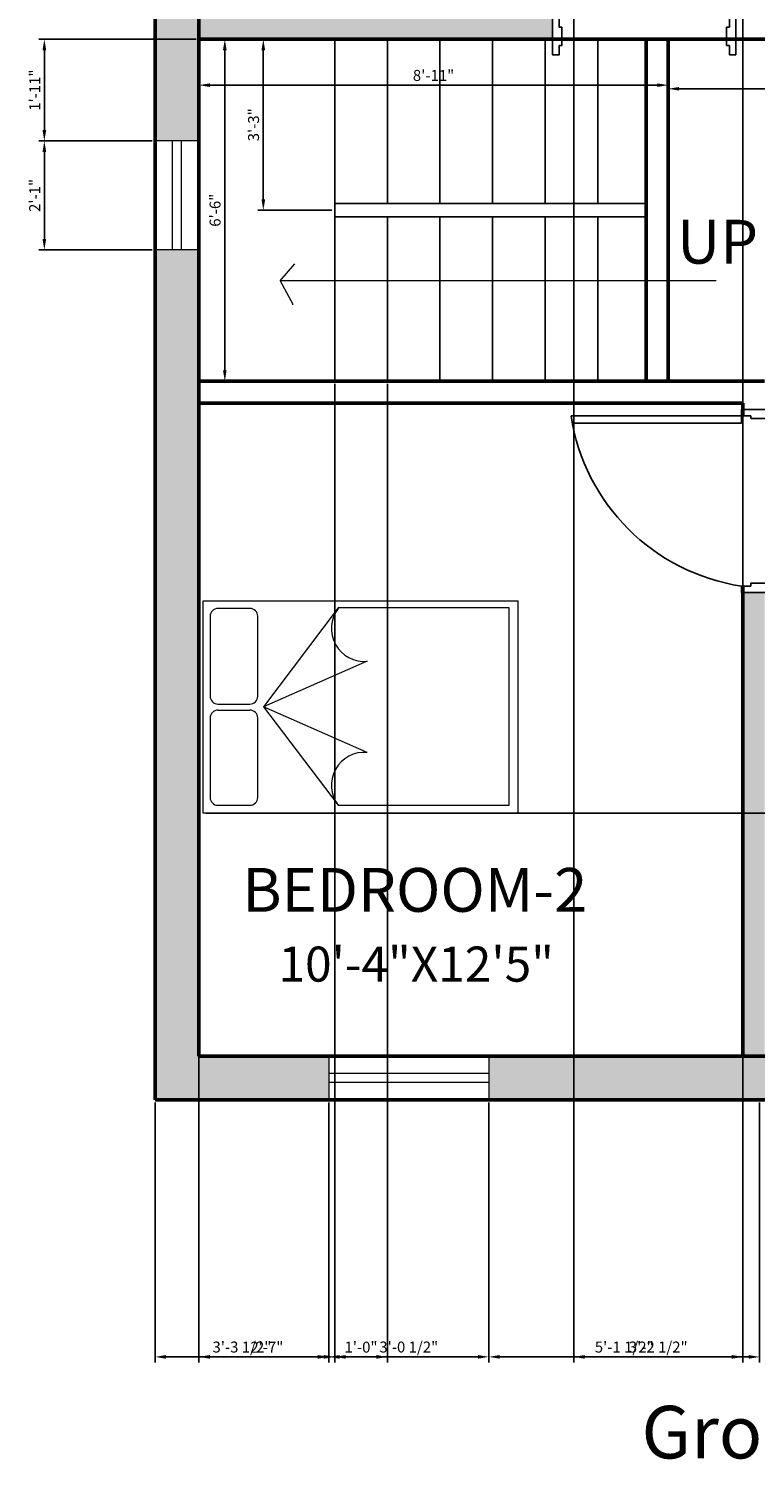
# Model space of a CAD drawing. Units: inches. Extents: x 3578 to 3951, y 1675 to 2189.
# Tile 1 of 4: x 3580 to 3746, y 1675 to 2001. Entities that reach past the tile are written whole.
import ezdxf

# ---------------------------------------------------------------- set-up
doc = ezdxf.new("R2010")
doc.units = ezdxf.units.IN
for name, color, linetype, lineweight in [('A-ANNO-DIMS', 2, 'Continuous', 18), ('A-ANNO-SYMB', 7, 'Continuous', 18), ('A-ANNO-TEXT', 7, 'Continuous', 25), ('A-AREA-IDEN', 7, 'Continuous', 25), ('A-DOOR', 3, 'Continuous', 25), ('A-FLOR-STRS', 7, 'Continuous', 25), ('A-FURN', 8, 'Continuous', 18), ('A-GLAZ', 4, 'Continuous', 18), ('A-WALL', 7, 'Continuous', 50), ('A-WALL-PATT', 8, 'Continuous', 13)]:
    doc.layers.add(name, color=color, linetype=linetype, lineweight=lineweight)
doc.styles.get("Standard").update_dxf_attribs({"font": 'arial.ttf'})
doc.dimstyles.new('ISO-25', dxfattribs={"dimtxt": 2.5, "dimasz": 2.5, "dimexe": 1.25, "dimexo": 0.625, "dimtad": 1, "dimdec": 0, "dimlunit": 4, "dimtxsty": 'Standard', "dimcen": 2.5, "dimadec": 0, "dimazin": 0, "dimtfac": 1, "dimtdec": 0, "dimtmove": 0, "dimatfit": 3, "dimfxl": 1, "dimarcsym": 0})

# ---------------------------------------------------------------- blocks, each defined once
blk = doc.blocks.new('A$C36772BAF')
for p, q in [((0, 0), (0, 2)), ((0, 2), (1.35, 2)), ((1.35, 2), (1.35, 0)), ((0.6051, 1.9554), (0.1004, 1.9554)), ((1.2508, 1.9554), (0.7437, 1.9554)), ((0.0504, 1.9054), (0.0504, 1.7024)), ((0.6551, 1.9054), (0.6551, 1.7024)), ((0.6937, 1.9054), (0.6937, 1.7024)), ((1.3008, 1.7024), (1.3008, 1.9054)), ((0.1004, 1.6524), (0.6051, 1.6524)), ((0.7437, 1.6524), (1.2508, 1.6524)), ((0.6756, 1.6168), (0.0504, 1.1415)), ((0.386, 0.9573), (0.6756, 1.6168)), ((0.9651, 0.9573), (0.6756, 1.6168)), ((1.305, 1.1415), (0.6756, 1.6168)), ((0.0504, 1.1415), (0.0504, 0.0572)), ((1.305, 0.0572), (1.305, 1.1415)), ((0, 0), (1.35, 0)), ((0.0504, 0.0572), (1.305, 0.0572))]:
    blk.add_line(p, q)
for centre, radius, start, end in [((0.1004, 1.9054), 0.05, 90, 180), ((0.6051, 1.9054), 0.05, 0, 90), ((0.7437, 1.9054), 0.05, 90, 180), ((1.2508, 1.9054), 0.05, 0, 90), ((0.1004, 1.7024), 0.05, 180, 270), ((0.6051, 1.7024), 0.05, 270, 0), ((0.7437, 1.7024), 0.05, 180, 270), ((1.2508, 1.7024), 0.05, 270, 0), ((0.1778, 0.9758), 0.2091, 354.93576, 127.55915), ((1.1733, 0.9758), 0.2091, 52.44085, 185.06424)]:
    blk.add_arc(centre, radius, start, end)
blk = doc.blocks.new('A$C40E8097C')
for p, q in [((33.6, 192), (33.6, 1074.8)), ((72, 192), (72, 1068.3)), ((0, 192), (0, 0)), ((33.6, 192), (0, 192)), ((33.6, 144), (33.6, 192)), ((48, 144), (33.6, 144)), ((48, 48), (48, 144)), ((33.6, 0), (33.6, 48)), ((33.6, 48), (48, 48)), ((0, 0), (33.6, 0))]:
    blk.add_line(p, q)
blk.add_lwpolyline([(33.6, 192), (72, 192)])
blk.add_lwpolyline([(950, 192), (950, 0), (916.4, 0), (916.4, 48), (902, 48), (902, 144), (916.4, 144), (916.4, 192)], close=True)
blk.add_arc((-123.6, 34.8), 1051.8, 8.59637, 81.40363)
blk = doc.blocks.new('*D8')
at = {"layer": 'A-ANNO-DIMS', "color": 0, "lineweight": -2, "transparency": 16777216}
for p, q in [((3619.18, 1998.14), (3619.18, 1987.06)), ((3726.18, 1998.14), (3726.18, 1987.06)), ((3621.68, 1988.31), (3723.68, 1988.31))]:
    blk.add_line(p, q, dxfattribs=at)
at = {"layer": 'A-ANNO-DIMS', "color": 0, "transparency": 16777216}
for points in [[(3621.68, 1988.72), (3621.68, 1987.89), (3619.18, 1988.31)], [(3723.68, 1988.72), (3723.68, 1987.89), (3726.18, 1988.31)]]:
    blk.add_solid(points, dxfattribs=at)
at = {"layer": 'Defpoints', "color": 0, "transparency": 16777216}
for p in [(3619.18, 1998.77), (3726.18, 1998.77), (3726.18, 1988.31)]:
    blk.add_point(p, dxfattribs=at)
at = {"layer": 'A-ANNO-DIMS', "color": 0, "transparency": 16777216, "insert": (3672.68, 1990.21), "char_height": 2.5, "attachment_point": 5}
blk.add_mtext('8\'-11"', dxfattribs=at)
blk = doc.blocks.new('*D9')
at = {"layer": 'A-ANNO-DIMS', "color": 0, "lineweight": -2, "transparency": 16777216}
for p, q in [((3649.51, 1998.77), (3632.61, 1998.77)), ((3633.86, 1996.27), (3633.86, 1962.27)), ((3649.51, 1959.77), (3632.61, 1959.77))]:
    blk.add_line(p, q, dxfattribs=at)
at = {"layer": 'A-ANNO-DIMS', "color": 0, "transparency": 16777216}
for points in [[(3633.44, 1996.27), (3634.28, 1996.27), (3633.86, 1998.77)], [(3633.44, 1962.27), (3634.28, 1962.27), (3633.86, 1959.77)]]:
    blk.add_solid(points, dxfattribs=at)
at = {"layer": 'Defpoints', "color": 0, "transparency": 16777216}
for p in [(3650.14, 1998.77), (3633.86, 1959.77), (3650.14, 1959.77)]:
    blk.add_point(p, dxfattribs=at)
at = {"layer": 'A-ANNO-DIMS', "color": 0, "transparency": 16777216, "insert": (3631.96, 1979.27), "char_height": 2.5, "attachment_point": 5, "rotation": 90}
blk.add_mtext('3\'-3"', dxfattribs=at)
blk = doc.blocks.new('*D10')
at = {"layer": 'A-ANNO-DIMS', "color": 0, "lineweight": -2, "transparency": 16777216}
for p, q in [((3619.8, 1998.77), (3626.33, 1998.77)), ((3625.08, 1996.27), (3625.08, 1923.27)), ((3619.8, 1920.77), (3626.33, 1920.77))]:
    blk.add_line(p, q, dxfattribs=at)
at = {"layer": 'A-ANNO-DIMS', "color": 0, "transparency": 16777216}
for points in [[(3624.66, 1996.27), (3625.5, 1996.27), (3625.08, 1998.77)], [(3624.66, 1923.27), (3625.5, 1923.27), (3625.08, 1920.77)]]:
    blk.add_solid(points, dxfattribs=at)
at = {"layer": 'Defpoints', "color": 0, "transparency": 16777216}
for p in [(3619.18, 1998.77), (3619.18, 1920.77), (3625.08, 1920.77)]:
    blk.add_point(p, dxfattribs=at)
at = {"layer": 'A-ANNO-DIMS', "color": 0, "transparency": 16777216, "insert": (3623.18, 1959.77), "char_height": 2.5, "attachment_point": 5, "rotation": 90}
blk.add_mtext('6\'-6"', dxfattribs=at)
blk = doc.blocks.new('*D12')
at = {"layer": 'A-ANNO-DIMS', "color": 0, "lineweight": -2, "transparency": 16777216}
for p, q in [((3726.18, 1987.68), (3726.18, 1986.23)), ((3728.68, 1987.48), (3821.68, 1987.48)), ((3824.18, 1987.68), (3824.18, 1986.23))]:
    blk.add_line(p, q, dxfattribs=at)
at = {"layer": 'A-ANNO-DIMS', "color": 0, "transparency": 16777216}
for points in [[(3728.68, 1987.9), (3728.68, 1987.07), (3726.18, 1987.48)], [(3821.68, 1987.9), (3821.68, 1987.07), (3824.18, 1987.48)]]:
    blk.add_solid(points, dxfattribs=at)
at = {"layer": 'Defpoints', "color": 0, "transparency": 16777216}
for p in [(3726.18, 1988.31), (3824.18, 1988.31), (3824.18, 1987.48)]:
    blk.add_point(p, dxfattribs=at)
at = {"layer": 'A-ANNO-DIMS', "color": 0, "transparency": 16777216, "insert": (3775.18, 1989.38), "char_height": 2.5, "attachment_point": 5}
blk.add_mtext('8\'-2"', dxfattribs=at)
blk = doc.blocks.new('*D29')
at = {"layer": 'A-ANNO-DIMS', "color": 0, "lineweight": -2, "transparency": 16777216}
for p, q in [((3618.55, 1998.77), (3582.68, 1998.77)), ((3583.93, 1996.27), (3583.93, 1978.07)), ((3608.55, 1975.57), (3582.68, 1975.57))]:
    blk.add_line(p, q, dxfattribs=at)
at = {"layer": 'A-ANNO-DIMS', "color": 0, "transparency": 16777216}
for points in [[(3583.51, 1996.27), (3584.35, 1996.27), (3583.93, 1998.77)], [(3583.51, 1978.07), (3584.35, 1978.07), (3583.93, 1975.57)]]:
    blk.add_solid(points, dxfattribs=at)
at = {"layer": 'Defpoints', "color": 0, "transparency": 16777216}
for p in [(3619.18, 1998.77), (3583.93, 1975.57), (3609.18, 1975.57)]:
    blk.add_point(p, dxfattribs=at)
at = {"layer": 'A-ANNO-DIMS', "color": 0, "transparency": 16777216, "insert": (3582.05, 1987.17), "char_height": 2.5, "attachment_point": 5, "rotation": 90}
blk.add_mtext('1\'-11"', dxfattribs=at)
blk = doc.blocks.new('*D30')
at = {"layer": 'A-ANNO-DIMS', "color": 0, "lineweight": -2, "transparency": 16777216}
for p, q in [((3608.55, 1975.57), (3582.68, 1975.57)), ((3583.93, 1973.07), (3583.93, 1953.21)), ((3608.55, 1950.71), (3582.68, 1950.71))]:
    blk.add_line(p, q, dxfattribs=at)
at = {"layer": 'A-ANNO-DIMS', "color": 0, "transparency": 16777216}
for points in [[(3583.51, 1973.07), (3584.35, 1973.07), (3583.93, 1975.57)], [(3583.51, 1953.21), (3584.35, 1953.21), (3583.93, 1950.71)]]:
    blk.add_solid(points, dxfattribs=at)
at = {"layer": 'Defpoints', "color": 0, "transparency": 16777216}
for p in [(3609.18, 1975.57), (3583.93, 1950.71), (3609.18, 1950.71)]:
    blk.add_point(p, dxfattribs=at)
at = {"layer": 'A-ANNO-DIMS', "color": 0, "transparency": 16777216, "insert": (3582.05, 1963.14), "char_height": 2.5, "attachment_point": 5, "rotation": 90}
blk.add_mtext('2\'-1"', dxfattribs=at)
blk = doc.blocks.new('*D37')
at = {"layer": 'A-ANNO-DIMS', "color": 0, "lineweight": -2, "transparency": 16777216}
for p, q in [((3609.18, 1756.14), (3609.18, 1696.88)), ((3648.78, 1756.14), (3648.78, 1696.88)), ((3611.68, 1698.13), (3646.28, 1698.13))]:
    blk.add_line(p, q, dxfattribs=at)
at = {"layer": 'A-ANNO-DIMS', "color": 0, "transparency": 16777216}
for points in [[(3611.68, 1698.55), (3611.68, 1697.71), (3609.18, 1698.13)], [(3646.28, 1698.55), (3646.28, 1697.71), (3648.78, 1698.13)]]:
    blk.add_solid(points, dxfattribs=at)
at = {"layer": 'Defpoints', "color": 0, "transparency": 16777216}
for p in [(3609.18, 1756.77), (3648.78, 1756.77), (3648.78, 1698.13)]:
    blk.add_point(p, dxfattribs=at)
at = {"layer": 'A-ANNO-DIMS', "color": 0, "transparency": 16777216, "insert": (3628.98, 1700.05), "char_height": 2.5, "attachment_point": 5}
blk.add_mtext('3\'-3 1/2"', dxfattribs=at)
blk = doc.blocks.new('*D38')
at = {"layer": 'A-ANNO-DIMS', "color": 0, "lineweight": -2, "transparency": 16777216}
for p, q in [((3648.78, 1756.14), (3648.78, 1696.88)), ((3685.29, 1756.14), (3685.29, 1696.88)), ((3651.28, 1698.13), (3682.79, 1698.13))]:
    blk.add_line(p, q, dxfattribs=at)
at = {"layer": 'A-ANNO-DIMS', "color": 0, "transparency": 16777216}
for points in [[(3651.28, 1698.55), (3651.28, 1697.71), (3648.78, 1698.13)], [(3682.79, 1698.55), (3682.79, 1697.71), (3685.29, 1698.13)]]:
    blk.add_solid(points, dxfattribs=at)
at = {"layer": 'Defpoints', "color": 0, "transparency": 16777216}
for p in [(3648.78, 1756.77), (3685.29, 1756.77), (3685.29, 1698.13)]:
    blk.add_point(p, dxfattribs=at)
at = {"layer": 'A-ANNO-DIMS', "color": 0, "transparency": 16777216, "insert": (3667.03, 1700.05), "char_height": 2.5, "attachment_point": 5}
blk.add_mtext('3\'-0 1/2"', dxfattribs=at)
blk = doc.blocks.new('*D39')
at = {"layer": 'A-ANNO-DIMS', "color": 0, "lineweight": -2, "transparency": 16777216}
for p, q in [((3685.29, 1756.14), (3685.29, 1696.88)), ((3747.04, 1756.14), (3747.04, 1696.88)), ((3687.79, 1698.13), (3744.54, 1698.13))]:
    blk.add_line(p, q, dxfattribs=at)
at = {"layer": 'A-ANNO-DIMS', "color": 0, "transparency": 16777216}
for points in [[(3687.79, 1698.55), (3687.79, 1697.71), (3685.29, 1698.13)], [(3744.54, 1698.55), (3744.54, 1697.71), (3747.04, 1698.13)]]:
    blk.add_solid(points, dxfattribs=at)
at = {"layer": 'Defpoints', "color": 0, "transparency": 16777216}
for p in [(3685.29, 1756.77), (3747.04, 1756.77), (3747.04, 1698.13)]:
    blk.add_point(p, dxfattribs=at)
at = {"layer": 'A-ANNO-DIMS', "color": 0, "transparency": 16777216, "insert": (3716.16, 1700.05), "char_height": 2.5, "attachment_point": 5}
blk.add_mtext('5\'-1 1/2"', dxfattribs=at)
blk = doc.blocks.new('*D49')
at = {"layer": 'A-ANNO-DIMS', "color": 0, "lineweight": -2, "transparency": 16777216}
for p, q in [((3619.18, 1920.14), (3619.18, 1696.88)), ((3650.14, 1920.14), (3650.14, 1696.88)), ((3621.68, 1698.13), (3647.64, 1698.13))]:
    blk.add_line(p, q, dxfattribs=at)
at = {"layer": 'A-ANNO-DIMS', "color": 0, "transparency": 16777216}
for points in [[(3621.68, 1698.55), (3621.68, 1697.71), (3619.18, 1698.13)], [(3647.64, 1698.55), (3647.64, 1697.71), (3650.14, 1698.13)]]:
    blk.add_solid(points, dxfattribs=at)
at = {"layer": 'Defpoints', "color": 0, "transparency": 16777216}
for p in [(3619.18, 1920.77), (3650.14, 1920.77), (3650.14, 1698.13)]:
    blk.add_point(p, dxfattribs=at)
at = {"layer": 'A-ANNO-DIMS', "color": 0, "transparency": 16777216, "insert": (3634.66, 1700.01), "char_height": 2.5, "attachment_point": 5}
blk.add_mtext('2\'-7"', dxfattribs=at)
blk = doc.blocks.new('*D50')
at = {"layer": 'A-ANNO-DIMS', "color": 0, "lineweight": -2, "transparency": 16777216}
for p, q in [((3650.14, 1920.14), (3650.14, 1696.88)), ((3662.14, 1920.14), (3662.14, 1696.88)), ((3652.64, 1698.13), (3659.64, 1698.13))]:
    blk.add_line(p, q, dxfattribs=at)
at = {"layer": 'A-ANNO-DIMS', "color": 0, "transparency": 16777216}
for points in [[(3652.64, 1698.55), (3652.64, 1697.71), (3650.14, 1698.13)], [(3659.64, 1698.55), (3659.64, 1697.71), (3662.14, 1698.13)]]:
    blk.add_solid(points, dxfattribs=at)
at = {"layer": 'Defpoints', "color": 0, "transparency": 16777216}
for p in [(3650.14, 1920.77), (3662.14, 1920.77), (3662.14, 1698.13)]:
    blk.add_point(p, dxfattribs=at)
at = {"layer": 'A-ANNO-DIMS', "color": 0, "transparency": 16777216, "insert": (3656.14, 1700.03), "char_height": 2.5, "attachment_point": 5}
blk.add_mtext('1\'-0"', dxfattribs=at)
blk = doc.blocks.new('*D54')
at = {"layer": 'A-ANNO-DIMS', "color": 0, "lineweight": -2, "transparency": 16777216}
for p, q in [((3704.64, 2107.33), (3704.64, 1696.88)), ((3743.18, 2098.14), (3743.18, 1696.88)), ((3740.68, 1698.13), (3707.14, 1698.13))]:
    blk.add_line(p, q, dxfattribs=at)
at = {"layer": 'A-ANNO-DIMS', "color": 0, "transparency": 16777216}
for points in [[(3707.14, 1698.55), (3707.14, 1697.71), (3704.64, 1698.13)], [(3740.68, 1698.55), (3740.68, 1697.71), (3743.18, 1698.13)]]:
    blk.add_solid(points, dxfattribs=at)
at = {"layer": 'Defpoints', "color": 0, "transparency": 16777216}
for p in [(3704.64, 2107.95), (3743.18, 2098.77), (3704.64, 1698.13)]:
    blk.add_point(p, dxfattribs=at)
at = {"layer": 'A-ANNO-DIMS', "color": 0, "transparency": 16777216, "insert": (3723.91, 1700.05), "char_height": 2.5, "attachment_point": 5}
blk.add_mtext('3\'-2 1/2"', dxfattribs=at)
blk = doc.blocks.new('*D57')
at = {"layer": 'A-ANNO-DIMS', "color": 0, "lineweight": -2, "transparency": 16777216}
for p, q in [((3620.74, 1822.18), (3936.33, 1822.18)), ((3935.08, 1769.27), (3935.08, 1819.68)), ((3619.8, 1766.77), (3936.33, 1766.77))]:
    blk.add_line(p, q, dxfattribs=at)
at = {"layer": 'A-ANNO-DIMS', "color": 0, "transparency": 16777216}
for points in [[(3934.66, 1819.68), (3935.5, 1819.68), (3935.08, 1822.18)], [(3934.66, 1769.27), (3935.5, 1769.27), (3935.08, 1766.77)]]:
    blk.add_solid(points, dxfattribs=at)
at = {"layer": 'Defpoints', "color": 0, "transparency": 16777216}
for p in [(3620.11, 1822.18), (3935.08, 1822.18), (3619.18, 1766.77)]:
    blk.add_point(p, dxfattribs=at)
at = {"layer": 'A-ANNO-DIMS', "color": 0, "transparency": 16777216, "insert": (3933.16, 1794.47), "char_height": 2.5, "attachment_point": 5, "rotation": 90}
blk.add_mtext('4\'-7 1/2"', dxfattribs=at)

msp = doc.modelspace()

# ---------------------------------------------------------------- hatches: boundary and pattern name
at = {"layer": 'A-WALL-PATT'}
h = msp.add_hatch(color=256, dxfattribs=at)
h.dxf.hatch_style = 1
h.paths.add_polyline_path([(3619.18, 1950.71), (3609.18, 1950.71), (3609.18, 1756.77), (3648.78, 1756.77), (3648.78, 1766.77), (3619.18, 1766.77)])
h.paths.add_polyline_path([(3619.18, 2068.71), (3609.18, 2068.71), (3609.18, 1975.57), (3619.18, 1975.57), (3619.18, 1998.77)])
h.paths.add_polyline_path([(3619.18, 2130.77), (3647.07, 2130.77), (3647.07, 2140.77), (3609.18, 2140.77), (3609.18, 2104.48), (3619.18, 2104.48)])
h.paths.add_polyline_path([(3909.18, 2140.77), (3713.13, 2140.77), (3713.13, 2130.77), (3899.18, 2130.77), (3899.18, 2110.42), (3909.18, 2110.42)])
h.paths.add_polyline_path([(3909.18, 2050.5), (3899.18, 2050.5), (3899.18, 1980.99), (3909.18, 1980.99)])
h.paths.add_polyline_path([(3909.18, 1881.86), (3899.18, 1881.86), (3899.18, 1941.89), (3890.7, 1942.45), (3889.21, 1942.68, -0.02009), (3881.89, 1944.66, -0.072677), (3876.18, 1946.94, -0.17277), (3874.16, 1950.75, -0.17277), (3875.79, 1954.64, -0.055418), (3880.27, 1956.72, -0.024581), (3889.21, 1959.22), (3890.7, 1959.45), (3899.18, 1960.01), (3899.18, 1952.98), (3909.18, 1952.98)])
h.paths.add_polyline_path([(3891.56, 1958.83, 0.100666), (3890.28, 1958.86, 0.024932), (3881.25, 1956.42, 0.064314), (3876.22, 1954.24, 0.17277), (3874.74, 1950.82, 0.17277), (3876.47, 1947.45, 0.072922), (3882.04, 1945.22, 0.022708), (3890.28, 1943.04, 0.100666), (3891.56, 1943.07, 0.125847)], flags=16)
h.paths.add_polyline_path([(3898.92, 1942.47, 0.324885), (3899.15, 1942.79), (3899.15, 1959.11, 0.551642), (3898.67, 1959.41), (3899.15, 1959.45), (3899.15, 1942.45)], flags=16)
h.paths.add_polyline_path([(3890.7, 1948.47, -1), (3891.63, 1948.47, -1)], flags=0)
h.paths.add_polyline_path([(3884.71, 1945.94, -0.104302), (3877.06, 1948.46, -0.17277), (3875.9, 1950.94, -0.17277), (3877.06, 1953.43, -0.104302), (3884.71, 1955.94, -0.414214), (3889.71, 1950.94, -0.414214)], flags=0)
h.paths.add_polyline_path([(3887.07, 1948.79), (3885.02, 1950.11, -0.031181), (3884.52, 1950.35, -0.229141), (3884.09, 1950.94, -0.229141), (3884.52, 1951.54, -0.109107), (3886.35, 1952.09, -0.199237), (3886.5, 1952.04, -0.461153), (3886.5, 1949.84), (3887.38, 1949.28)], flags=0)
h.paths.add_polyline_path([(3890.7, 1953.43, -1), (3891.63, 1953.43, -1)], flags=0)
h.paths.add_polyline_path([(3909.18, 1843.84), (3899.18, 1843.84), (3899.18, 1766.77), (3844.49, 1766.77), (3844.49, 1756.77), (3909.18, 1756.77)])
h = msp.add_hatch(color=256, dxfattribs=at)
h.dxf.hatch_style = 1
h.paths.add_polyline_path([(3899.18, 2003.77), (3789.71, 2003.77, -0.003692), (3789.81, 2003.09), (3791.29, 2003.09), (3791.29, 1998.77), (3899.18, 1998.77)])
h.paths.add_polyline_path([(3748.18, 2130.77), (3743.18, 2130.77), (3743.18, 2003.77), (3748.18, 2003.77)])
h.paths.add_polyline_path([(3899.18, 1920.77), (3864.53, 1920.77), (3864.53, 1915.77), (3899.18, 1915.77)], flags=0)
h.paths.add_polyline_path([(3748.18, 1872.53), (3743.18, 1872.53), (3743.18, 1766.77), (3748.18, 1766.77)], flags=0)
h.paths.add_polyline_path([(3807.15, 1834.35), (3847.1, 1834.35), (3847.1, 1854.95), (3807.15, 1854.95)], flags=8)
h.paths.add_polyline_path([(3791.36, 1816.7), (3859.75, 1816.7), (3859.75, 1833.18), (3791.36, 1833.18)], flags=8)
h.paths.add_polyline_path([(3771.09, 1986.79), (3779.29, 1986.79), (3779.29, 1991.94), (3771.09, 1991.94)], flags=8)
h.paths.add_polyline_path([(3782.02, 1935.64), (3790.22, 1935.64), (3790.22, 1940.79), (3782.02, 1940.79)], flags=8)
h = msp.add_hatch(color=256, dxfattribs=at)
h.dxf.hatch_style = 1
h.paths.add_polyline_path([(3748.18, 1872.53), (3743.18, 1872.53), (3743.18, 1766.77), (3748.18, 1766.77)], flags=0)
h.paths.add_polyline_path([(3815.97, 1920.2), (3822.72, 1920.2), (3822.72, 1920.6), (3824.18, 1920.6), (3824.18, 1998.77), (3791.29, 1998.77), (3791.29, 1994.64), (3789.81, 1994.64), (3789.81, 1996.75), (3789.18, 1996.75), (3789.18, 1998.77), (3751.6, 1998.77), (3751.6, 1996.75), (3750.96, 1996.75), (3750.96, 1994.64), (3749.49, 1994.64), (3749.49, 1998.77), (3741.62, 1998.77), (3741.62, 1995.21), (3740.14, 1995.21), (3740.14, 1997.32), (3739.51, 1997.32), (3739.51, 1998.77), (3726.18, 1998.77), (3726.18, 1920.73), (3726.07, 1920.73), (3619.18, 1920.77), (3619.18, 1915.77), (3743.18, 1915.77), (3743.18, 1914.33), (3751.33, 1914.33), (3751.33, 1912.86), (3749.22, 1912.86), (3749.22, 1912.22), (3745, 1912.22), (3745, 1912.86), (3742.88, 1912.86), (3742.88, 1911.17), (3704.32, 1911.17, 0.31859), (3742.88, 1874.01), (3745, 1874.01), (3745, 1874.64), (3749.22, 1874.64), (3749.22, 1874.01), (3751.33, 1874.01), (3751.33, 1872.53), (3748.18, 1872.53), (3748.18, 1766.77), (3751.55, 1766.77), (3751.55, 1767.57), (3753.03, 1767.57), (3753.03, 1806.42, -0.328818), (3791.88, 1767.57), (3793.35, 1767.57), (3793.35, 1766.77), (3899.18, 1766.77), (3899.18, 1915.77), (3864.53, 1915.77), (3864.53, 1912.15), (3863.05, 1912.15), (3863.05, 1914.26), (3862.42, 1914.26), (3862.42, 1915.77), (3824.84, 1915.77), (3824.84, 1914.26), (3824.2, 1914.26), (3824.2, 1912.15), (3822.72, 1912.15), (3822.72, 1915.77), (3815.97, 1915.77)], flags=17)
h.paths.add_polyline_path([(3815.97, 1920.2), (3822.72, 1920.2), (3822.72, 1920.6), (3824.18, 1920.6), (3824.18, 1998.77), (3791.29, 1998.77), (3791.29, 1994.64), (3789.81, 1994.64), (3789.81, 1996.75), (3789.18, 1996.75), (3789.18, 1998.77), (3751.6, 1998.77), (3751.6, 1996.75), (3750.96, 1996.75), (3750.96, 1994.64), (3749.49, 1994.64), (3749.49, 1998.77), (3741.62, 1998.77), (3741.62, 1995.21), (3740.14, 1995.21), (3740.14, 1997.32), (3739.51, 1997.32), (3739.51, 1998.77), (3726.18, 1998.77), (3726.18, 1920.73), (3619.18, 1920.77), (3619.18, 1915.77), (3743.18, 1915.77), (3743.18, 1914.33), (3751.33, 1914.33), (3751.33, 1912.86), (3749.22, 1912.86), (3749.22, 1912.22), (3745, 1912.22), (3745, 1912.86), (3742.88, 1912.86), (3742.88, 1911.17), (3704.32, 1911.17, 0.31859), (3742.88, 1874.01), (3745, 1874.01), (3745, 1874.64), (3749.22, 1874.64), (3749.22, 1874.01), (3751.33, 1874.01), (3751.33, 1872.53), (3748.18, 1872.53), (3748.18, 1766.77), (3751.55, 1766.77), (3751.55, 1767.57), (3753.03, 1767.57), (3753.03, 1806.42, -0.328818), (3791.88, 1767.57), (3793.35, 1767.57), (3793.35, 1766.77), (3899.18, 1766.77), (3899.18, 1915.77), (3864.53, 1915.77), (3864.53, 1912.15), (3863.05, 1912.15), (3863.05, 1914.26), (3862.42, 1914.26), (3862.42, 1915.77), (3824.84, 1915.77), (3824.84, 1914.26), (3824.2, 1914.26), (3824.2, 1912.15), (3822.72, 1912.15), (3822.72, 1915.77), (3815.97, 1915.77)], flags=17)
h.paths.add_polyline_path([(3699.81, 2003.77), (3619.18, 2003.77), (3619.18, 1998.77), (3699.81, 1998.77)])
h.paths.add_polyline_path([(3807.15, 1834.35), (3847.1, 1834.35), (3847.1, 1854.95), (3807.15, 1854.95)], flags=8)
h.paths.add_polyline_path([(3791.36, 1816.7), (3859.75, 1816.7), (3859.75, 1833.18), (3791.36, 1833.18)], flags=8)
h = msp.add_hatch(color=256, dxfattribs=at)
h.dxf.hatch_style = 1
h.paths.add_polyline_path([(3748.18, 1872.53), (3743.18, 1872.53), (3743.18, 1766.77), (3748.18, 1766.77)])
h = msp.add_hatch(color=256, dxfattribs=at)
h.dxf.hatch_style = 1
h.paths.add_polyline_path([(3791.24, 1765.45), (3791.88, 1765.45), (3791.88, 1766.77), (3753.03, 1766.77), (3753.03, 1765.45), (3753.66, 1765.45), (3753.66, 1761.23), (3753.03, 1761.23), (3753.03, 1759.12), (3751.55, 1759.12), (3751.55, 1766.77), (3685.29, 1766.77), (3685.29, 1756.77), (3822.14, 1756.77), (3822.14, 1766.77), (3793.35, 1766.77), (3793.35, 1759.12), (3791.88, 1759.12), (3791.88, 1761.23), (3791.24, 1761.23)])

# ---------------------------------------------------------------- linework, layer by layer
at = {"layer": 'A-ANNO-SYMB'}
for p, q in [((3637.73, 1943.63), (3641.06, 1947.56)), ((3737.15, 1943.63), (3637.73, 1943.63)), ((3637.73, 1943.63), (3640.61, 1938.33)), ((3640.61, 1938.15), (3640.61, 1938.33))]:
    msp.add_line(p, q, dxfattribs=at)
at = {"layer": 'A-FLOR-STRS'}
for p, q in [((3650.14, 1998.77), (3650.14, 1961.27)), ((3650.14, 1998.77), (3650.14, 1959.77)), ((3650.14, 1998.77), (3650.14, 1958.27)), ((3662.14, 1998.77), (3662.14, 1961.27)), ((3674.14, 1998.77), (3674.14, 1961.27)), ((3686.14, 1998.77), (3686.14, 1961.27)), ((3698.14, 1998.77), (3698.14, 1961.27)), ((3710.14, 1998.77), (3710.14, 1961.27)), ((3650.14, 1961.27), (3721.14, 1961.27)), ((3650.14, 1958.27), (3721.14, 1958.27)), ((3650.14, 1958.27), (3650.14, 1920.77)), ((3662.14, 1958.27), (3662.14, 1920.77)), ((3674.14, 1958.27), (3674.14, 1920.77)), ((3686.14, 1958.27), (3686.14, 1920.77)), ((3698.14, 1958.27), (3698.14, 1920.77)), ((3710.14, 1958.27), (3710.14, 1920.77))]:
    msp.add_line(p, q, dxfattribs=at)
at = {"layer": 'A-GLAZ'}
for p, q in [((3619.18, 1975.57), (3609.18, 1975.57)), ((3613.18, 1950.71), (3613.18, 1975.57)), ((3615.18, 1950.71), (3615.18, 1975.57)), ((3619.18, 1950.71), (3609.18, 1950.71)), ((3648.78, 1766.77), (3648.78, 1756.77)), ((3685.29, 1766.77), (3685.29, 1756.77)), ((3685.29, 1762.77), (3648.78, 1762.77)), ((3685.29, 1760.77), (3648.78, 1760.77))]:
    msp.add_line(p, q, dxfattribs=at)
at = {"layer": 'A-WALL'}
for p, q in [((3609.18, 1756.77), (3609.18, 2140.77)), ((3619.18, 1766.77), (3619.18, 2130.77)), ((3619.18, 1998.77), (3899.18, 1998.77)), ((3619.18, 1998.77), (3619.18, 1920.77)), ((3619.18, 1998.77), (3619.18, 1920.77)), ((3619.18, 1998.77), (3726.18, 1998.77)), ((3721.14, 1920.77), (3721.14, 1998.77)), ((3726.14, 1920.77), (3726.14, 1998.77)), ((3726.18, 1998.77), (3726.18, 1920.77)), ((3619.18, 1920.77), (3726.18, 1920.77)), ((3726.07, 1920.73), (3748.16, 1920.73)), ((3619.18, 1915.77), (3743.18, 1915.77)), ((3743.18, 1912.86), (3743.18, 1915.77)), ((3743.18, 1915.73), (3743.18, 1915.77)), ((3743.18, 1766.77), (3743.18, 1874.01)), ((3619.18, 1766.77), (3743.18, 1766.77)), ((3619.18, 1766.77), (3743.18, 1766.77)), ((3753.03, 1766.77), (3619.18, 1766.77)), ((3909.18, 1756.77), (3609.18, 1756.77))]:
    msp.add_line(p, q, dxfattribs=at)

# ---------------------------------------------------------------- block references
at = {"layer": 'A-DOOR', "xscale": -0.044006868052547, "yscale": 0.044006868052547, "zscale": 0.044006868052547}
msp.add_blockref('A$C40E8097C', (3741.62, 1995.21), dxfattribs=at)
at = {"layer": 'A-DOOR', "xscale": -0.044006868052547, "yscale": 0.044006868052547, "zscale": 0.044006868052547, "rotation": 90}
msp.add_blockref('A$C40E8097C', (3751.33, 1914.33), dxfattribs=at)
at = {"layer": 'A-FURN', "xscale": 35.91900852829305, "yscale": 35.91900852829305, "zscale": 35.91900852829305, "rotation": 90}
msp.add_blockref('A$C36772BAF', (3691.95, 1822.18), dxfattribs=at)

# ---------------------------------------------------------------- texts
at = {"layer": 'A-ANNO-TEXT', "attachment_point": 1}
for s, insert, char_height in [('UP', (3728.21, 1957.59), 10), ('Ground Floor Plan', (3720.09, 1686.95), 12)]:
    msp.add_mtext(s, dxfattribs=dict(at, insert=insert, char_height=char_height))
at = {"layer": 'A-AREA-IDEN', "attachment_point": 1}
for s, insert, char_height in [('BEDROOM-2', (3629.07, 1809.69), 10), ('10\'-4"X12\'5"', (3637.32, 1791.75), 8)]:
    msp.add_mtext(s, dxfattribs=dict(at, insert=insert, char_height=char_height))

# ---------------------------------------------------------------- dimensions: what is measured, and where the dimension line sits
at = {"layer": 'A-ANNO-DIMS'}
for base, p1, p2, override, picture, middle in [((3704.64, 1698.13), (3743.18, 2098.77), (3704.64, 2107.95), {"dimdec": 1, "dimlfac": 1, "dimrnd": 0, "dimzin": 1, "dimdsep": 46, "dimlunit": 4, "dimfrac": 2}, '*D54', (3723.91, 1700.05)), ((3726.18, 1988.31), (3619.18, 1998.77), (3726.18, 1998.77), {"dimclrd": 0, "dimclre": 0, "dimclrt": 0}, '*D8', (3672.68, 1990.21)), ((3824.18, 1987.48), (3726.18, 1988.31), (3824.18, 1988.31), {"dimclrd": 0, "dimclre": 0, "dimclrt": 0}, '*D12', (3775.18, 1989.38)), ((3650.14, 1698.13), (3619.18, 1920.77), (3650.14, 1920.77), {"dimdec": 1, "dimlfac": 1, "dimrnd": 0, "dimzin": 1, "dimdsep": 46, "dimlunit": 4, "dimfrac": 2}, '*D49', (3634.66, 1700.01)), ((3662.14, 1698.13), (3650.14, 1920.77), (3662.14, 1920.77), {"dimdec": 1, "dimlfac": 1, "dimrnd": 0, "dimzin": 1, "dimdsep": 46, "dimlunit": 4, "dimfrac": 2}, '*D50', (3656.14, 1700.03)), ((3648.78, 1698.13), (3609.18, 1756.77), (3648.78, 1756.77), {"dimdec": 1, "dimlfac": 1, "dimrnd": 0, "dimzin": 1, "dimdsep": 46, "dimlunit": 4, "dimfrac": 2}, '*D37', (3628.98, 1700.05)), ((3685.29, 1698.13), (3648.78, 1756.77), (3685.29, 1756.77), {"dimdec": 1, "dimlfac": 1, "dimrnd": 0, "dimzin": 1, "dimdsep": 46, "dimlunit": 4, "dimfrac": 2}, '*D38', (3667.03, 1700.05)), ((3747.0353, 1698.131), (3685.288, 1756.7652), (3747.0353, 1756.7652), {"dimdec": 1, "dimlfac": 1, "dimrnd": 0, "dimzin": 1, "dimdsep": 46, "dimlunit": 4, "dimfrac": 2}, '*D39', (3716.1617, 1700.0486))]:
    dim = msp.add_linear_dim(base=base, p1=p1, p2=p2, dimstyle='ISO-25', override=override, dxfattribs=at)
    dim.commit()
    dim.dimension.update_dxf_attribs({"geometry": picture, "text_midpoint": middle})
for base, p1, p2, override, picture, middle in [((3583.93, 1975.57), (3619.18, 1998.77), (3609.18, 1975.57), {"dimdec": 1, "dimlfac": 1, "dimrnd": 0, "dimzin": 1, "dimdsep": 46, "dimlunit": 4, "dimfrac": 2}, '*D29', (3582.05, 1987.17)), ((3625.08, 1920.77), (3619.18, 1998.77), (3619.18, 1920.77), {"dimclrd": 0, "dimclre": 0, "dimclrt": 0}, '*D10', (3623.18, 1959.77)), ((3633.86, 1959.77), (3650.14, 1998.77), (3650.14, 1959.77), {"dimclrd": 0, "dimclre": 0, "dimclrt": 0}, '*D9', (3631.96, 1979.27)), ((3583.93, 1950.71), (3609.18, 1975.57), (3609.18, 1950.71), {"dimdec": 1, "dimlfac": 1, "dimrnd": 0, "dimzin": 1, "dimdsep": 46, "dimlunit": 4, "dimfrac": 2}, '*D30', (3582.05, 1963.14)), ((3935.08, 1822.18), (3619.18, 1766.77), (3620.11, 1822.18), {"dimdec": 1, "dimlfac": 1, "dimrnd": 0, "dimzin": 1, "dimdsep": 46, "dimlunit": 4, "dimfrac": 2}, '*D57', (3933.16, 1794.47))]:
    dim = msp.add_linear_dim(base=base, p1=p1, p2=p2, angle=90, dimstyle='ISO-25', override=override, dxfattribs=at)
    dim.commit()
    dim.dimension.update_dxf_attribs({"geometry": picture, "text_midpoint": middle})

doc.saveas('drawing.dxf')
